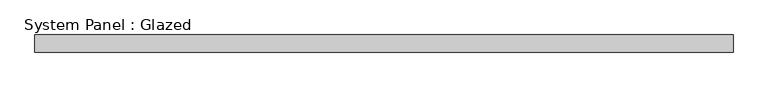
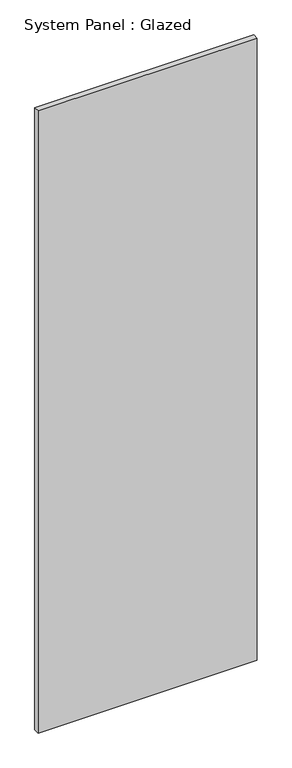
"""IFC4 building model written with IfcOpenShell, lengths in millimetres: plate geometry, System Panel : Glazed."""

from ifc_helpers import new_model, si_unit, origin, origin_with_axes, place, context, project, spatial, polyline, outline, extrude, source, transform, mapped, element, save


def system_panel_glazed_00cb815b(model_context):
    return source(origin(), model_context, "Body", "SweptSolid", [
        extrude(outline(polyline([(508.0, 19.05), (-508.0, 19.05), (-508.0, 44.45), (508.0, 44.45), (508.0, 19.05)])), origin_with_axes(), (0.0, 0.0, 1.0), 3048.0),
    ])


if __name__ == "__main__":
    model = new_model("IFC4")
    model_context = context("Model", 3, world=origin())
    ifc_project = project(units=[si_unit("LENGTHUNIT", "METRE", prefix="MILLI")], contexts=[model_context])
    site = spatial("IfcSite", under=ifc_project)
    building = spatial("IfcBuilding", under=site)
    placement = place(None, origin())
    system_panel_glazed_shape = system_panel_glazed_00cb815b(model_context)
    element("IfcPlate", 1, ObjectType="System Panel : Glazed", at=placement, inside=building, context=model_context, shape_type="MappedRepresentation", body=[
        mapped(system_panel_glazed_shape, transform((0.0, 0.0, 0.0), x_axis=(1.0, 0.0, 0.0), y_axis=(0.0, 1.0, 0.0), z_axis=(0.0, 0.0, 1.0))),
    ])
    save(model, "model.ifc")

# Revit data of these elements
# Type "System Panel : Glazed"
#   Construction Type Id = "GSP4R"
#   Analytic Construction = "1/8 in Pilkington single glazing"
#   Visual Light Transmittance = 0.9
#   Solar Heat Gain Coefficient = 0.86
#   Heat Transfer Coefficient (U) = 1.18115 BTU/(h·ft²·°F)
# Element 1 (IfcPlate, "System Panel : Glazed")
#   Materials on its faces: "Glass"
# Materials
#   "Glass": class "Glass", colour RGB 0 128 192, transparency 0.75, Description = "Soda Lime Glass", Cost = 0
